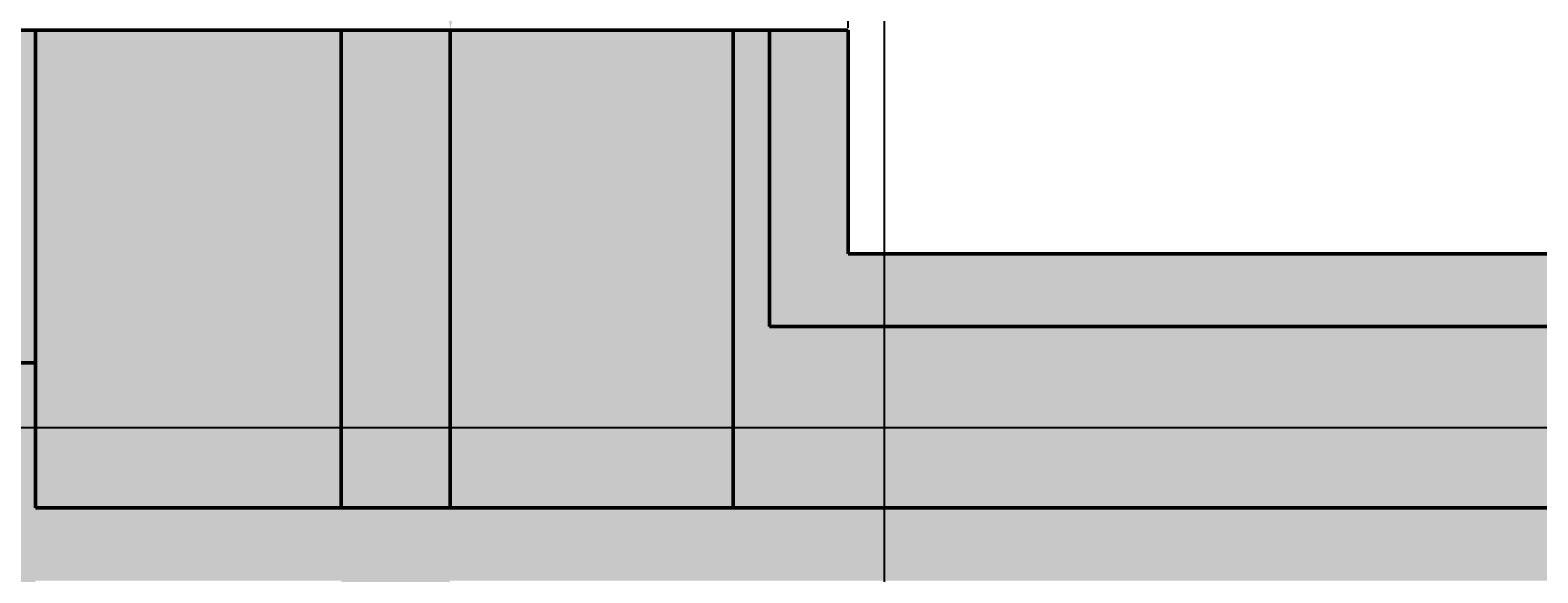
# Model space of a CAD drawing. Units: inches. Extents: x -12 to 334, y -10 to 186.
# Tile 19 of 77: x 64 to 106, y 94 to 109. Entities that reach past the tile are written whole.
import ezdxf
from ezdxf import colors
from ezdxf.entities.mleader import LeaderData, LeaderLine
from ezdxf.math import Vec2, Vec3

# ---------------------------------------------------------------- set-up
doc = ezdxf.new("R2010")
doc.units = ezdxf.units.IN
doc.header["$MEASUREMENT"] = 0
for name, color, linetype, lineweight in [('M-ANNO-TEXT', 3, 'Continuous', 25), ('M-DIMS', 2, 'Continuous', 18), ('M-EQPM', 7, 'Continuous', 50), ('M-EQPM-PATT', 8, 'Continuous', 18)]:
    doc.layers.add(name, color=color, linetype=linetype, lineweight=lineweight)
doc.styles.get("Standard").update_dxf_attribs({"font": 'arial.ttf'})
doc.dimstyles.get("Standard").update_dxf_attribs({"dimtxt": 0.18, "dimasz": 0.18, "dimexe": 0.18, "dimexo": 0.0625, "dimgap": 0.09, "dimtad": 0, "dimtih": 1, "dimtoh": 1, "dimdec": 4, "dimzin": 0, "dimdsep": 46, "dimtxsty": 'Standard', "dimcen": 0.09, "dimadec": 0, "dimazin": 0, "dimtfac": 1, "dimtdec": 4, "dimtofl": 0, "dimtmove": 0, "dimatfit": 3, "dimfxl": 1, "dimtolj": 1, "dimtzin": 0, "dimarcsym": 0})

# ---------------------------------------------------------------- blocks, each defined once
blk = doc.blocks.new('*D15')
at = {"layer": 'Defpoints', "color": 0, "transparency": 16777216}
for p in [(106.177, 169.385), (86.888, 109.058), (106.177, 102.896)]:
    blk.add_point(p, dxfattribs=at)
at = {"layer": 'M-DIMS', "color": 0, "lineweight": -2, "transparency": 16777216}
for p, q in [((86.888, 109.121), (86.888, 169.565)), ((106.177, 102.958), (106.177, 169.565)), ((87.068, 169.385), (96.147, 169.385)), ((105.997, 169.385), (96.918, 169.385))]:
    blk.add_line(p, q, dxfattribs=at)
at = {"layer": 'M-DIMS', "color": 0, "transparency": 16777216}
for points in [[(87.068, 169.415), (87.068, 169.355), (86.888, 169.385)], [(105.997, 169.415), (105.997, 169.355), (106.177, 169.385)]]:
    blk.add_solid(points, dxfattribs=at)
at = {"layer": 'M-DIMS', "color": 0, "transparency": 16777216, "insert": (96.532, 169.385), "char_height": 0.18, "attachment_point": 5}
blk.add_mtext('\\A1;19.29', dxfattribs=at)
blk = doc.blocks.new('*D26')
at = {"layer": 'Defpoints', "color": 0, "transparency": 16777216}
for p in [(87.888, 169.385), (87.888, 56.321), (58.1, 33.675)]:
    blk.add_point(p, dxfattribs=at)
at = {"layer": 'M-DIMS', "color": 0, "lineweight": -2, "transparency": 16777216}
for p, q in [((58.1, 33.738), (58.1, 169.565)), ((87.888, 56.383), (87.888, 169.565)), ((58.28, 169.385), (72.599, 169.385)), ((87.708, 169.385), (73.389, 169.385))]:
    blk.add_line(p, q, dxfattribs=at)
at = {"layer": 'M-DIMS', "color": 0, "transparency": 16777216}
for points in [[(58.28, 169.415), (58.28, 169.355), (58.1, 169.385)], [(87.708, 169.415), (87.708, 169.355), (87.888, 169.385)]]:
    blk.add_solid(points, dxfattribs=at)
at = {"layer": 'M-DIMS', "color": 0, "transparency": 16777216, "insert": (72.994, 169.385), "char_height": 0.18, "attachment_point": 5}
blk.add_mtext('\\A1;29.79', dxfattribs=at)
blk = doc.blocks.new('*D35')
at = {"layer": 'Defpoints', "color": 0, "transparency": 16777216}
for p in [(216.428, 98.108), (-11.174, 61.105), (216.428, 61.105)]:
    blk.add_point(p, dxfattribs=at)
at = {"layer": 'M-DIMS', "color": 0, "lineweight": -2, "transparency": 16777216}
for p, q in [((216.365, 98.108), (-11.354, 98.108)), ((-11.174, 97.928), (-11.174, 79.788)), ((-11.174, 61.285), (-11.174, 79.424)), ((216.365, 61.105), (-11.354, 61.105))]:
    blk.add_line(p, q, dxfattribs=at)
at = {"layer": 'M-DIMS', "color": 0, "transparency": 16777216}
for points in [[(-11.204, 97.928), (-11.144, 97.928), (-11.174, 98.108)], [(-11.204, 61.285), (-11.144, 61.285), (-11.174, 61.105)]]:
    blk.add_solid(points, dxfattribs=at)
at = {"layer": 'M-DIMS', "color": 0, "transparency": 16777216, "insert": (-11.174, 79.606), "char_height": 0.18, "attachment_point": 5}
blk.add_mtext('\\A1;37', dxfattribs=at)

msp = doc.modelspace()

# ---------------------------------------------------------------- hatches: boundary and pattern name
at = {"layer": 'M-EQPM-PATT'}
h = msp.add_hatch(color=256, dxfattribs=at)
h.set_gradient(color1=(99, 100, 102), color2=(99, 100, 102), tint=1)
h.paths.add_polyline_path([(126.9567, 136.8871), (179.7818, 136.8871), (180.0106, 137.8871), (126.3793, 137.8871), (106.1771, 102.8958), (86.8879, 102.8958), (86.8879, 109.0583), (84.7229, 109.0583), (84.7229, 100.8958), (106.1771, 100.8958)])
h.paths.add_polyline_path([(196.3421, 152.8345), (195.3421, 152.8345), (195.3421, 137.8871), (180.0106, 137.8871), (179.7818, 136.8871), (196.3421, 136.8871)])
h.paths.add_polyline_path([(215.0166, 152.8345), (214.0166, 152.8345), (214.0166, 136.9435), (268.3808, 136.9435, -0.2673785), (268.3808, 46.8541), (249.3759, 46.8541), (249.8485, 45.8541), (269.3808, 45.8541, 0.2615891), (269.3808, 137.9435), (215.0166, 137.9435)])
h = msp.add_hatch(color=256, dxfattribs=at)
h.set_gradient(color1=(99, 100, 102), color2=(99, 100, 102), tint=1)
h.paths.add_polyline_path([(4.3766, 80.754, -0.4132606), (23.5807, 99.8958), (37.1002, 99.8958), (37.1002, 127.7078), (32.1002, 127.7078), (32.1002, 125.2078), (36.1002, 125.2078), (36.1002, 100.8958), (23.5807, 100.8958, 1), (23.5807, 60.4872), (36.1002, 60.4872), (36.1002, 36.1752), (32.1002, 36.1752), (32.1002, 33.6752), (37.1002, 33.6752), (37.1002, 61.4872), (23.5807, 61.4872, -0.384914), (4.4744, 78.754), (72.9244, 78.754), (72.9244, 69.6117), (75.9244, 69.6117), (75.9244, 89.8963), (72.9244, 89.8963), (72.9244, 80.754)])
h.paths.add_polyline_path([(54.1002, 125.2078), (58.1002, 125.2078), (58.1002, 127.7078), (53.1002, 127.7078), (53.1002, 99.8958), (64.5, 99.8958), (64.5, 109.0583), (63.5, 109.0583), (63.5, 100.8958), (54.1002, 100.8958)], flags=17)
h.paths.add_polyline_path([(53.1002, 33.6752), (58.1002, 33.6752), (58.1002, 36.1752), (54.1002, 36.1752), (54.1002, 60.4872), (64.2068, 60.4872), (64.2068, 49.4497), (87.8879, 49.4497), (87.8879, 55.3205), (104.8919, 55.3205), (104.8919, 30.8541), (99.8919, 30.8541), (99.8919, 28.8541), (105.8919, 28.8541), (105.8919, 56.3205), (87.8879, 56.3205), (87.8879, 63.6117), (86.8879, 63.6117), (86.8879, 50.4497), (65.0061, 50.4497), (65.0061, 63.6117), (64.5, 63.6117), (64.5, 61.4872), (53.1002, 61.4872)])
h.paths.add_polyline_path([(121.8919, 28.8541), (121.8919, 30.8541), (116.8919, 30.8541), (116.8919, 45.8541), (209.6965, 45.8541), (209.9204, 46.8541), (115.8919, 46.8541), (115.8919, 28.8541)])
h.paths.add_polyline_path([(221.5761, 32.8541), (216.5761, 32.8541), (216.5761, 30.8541), (222.5761, 30.8541), (222.5761, 46.8541), (209.9204, 46.8541), (209.6965, 45.8541), (221.5761, 45.8541)])
h.paths.add_polyline_path([(233.5761, 45.8541), (249.8485, 45.8541), (249.3759, 46.8541), (232.5761, 46.8541), (232.5761, 30.8541), (238.5761, 30.8541), (238.5761, 32.8541), (233.5761, 32.8541)])
h = msp.add_hatch(color=256, dxfattribs=at)
h.set_gradient(color1=(205, 32, 39), color2=(205, 32, 39), tint=1)
h.paths.add_polyline_path([(64.5, 80.754), (64.5, 89.8963), (226.6083, 89.8963, -1), (226.6083, 69.6117), (64.5, 69.6117), (64.5, 78.754), (4.4744, 78.754, 0.384914), (23.5807, 61.4872), (37.1002, 61.4872), (37.1002, 33.6752), (53.1002, 33.6752), (53.1002, 61.4872), (64.5, 61.4872), (64.5, 63.6117), (226.6083, 63.6117, 1), (226.6083, 95.8963), (64.5, 95.8963), (64.5, 99.8958), (53.1002, 99.8958), (53.1002, 127.7078), (37.1002, 127.7078), (37.1002, 99.8958), (23.5807, 99.8958, 0.4132606), (4.3766, 80.754)])
h.paths.add_polyline_path([(64.5, 91.8963), (64.5, 93.8963), (226.6083, 93.8963, -1), (226.6083, 65.6117), (64.5, 65.6117), (64.5, 67.6117), (226.6083, 67.6117, 1), (226.6083, 91.8963)], flags=16)
h = msp.add_hatch(color=256, dxfattribs=at)
h.set_gradient(color1=(205, 32, 39), color2=(205, 32, 39), tint=1)
h.paths.add_polyline_path([(72.9244, 95.8963), (72.9244, 109.0583), (64.5, 109.0583), (64.5, 95.8963)])
h.paths.add_polyline_path([(72.9244, 80.754), (72.9244, 89.8963), (64.5, 89.8963), (64.5, 80.754)])
h.paths.add_polyline_path([(72.9244, 69.6117), (72.9244, 78.754), (64.5, 78.754), (64.5, 69.6117)])
h.paths.add_polyline_path([(72.9244, 50.4497), (72.9244, 63.6117), (65.0061, 63.6117), (65.0061, 50.4497)])
h = msp.add_hatch(color=256, dxfattribs=at)
h.set_gradient(color1=(99, 100, 102), color2=(99, 100, 102), tint=1)
h.paths.add_polyline_path([(72.9244, 95.8963), (75.9244, 95.8963), (75.9244, 109.0583), (72.9244, 109.0583)])
h.paths.add_polyline_path([(72.9244, 50.4497), (75.9244, 50.4497), (75.9244, 63.6117), (72.9244, 63.6117)])
h.paths.add_polyline_path([(75.9244, 91.8963), (75.9244, 93.8963), (72.9244, 93.8963), (72.9244, 91.8963)])
h.paths.add_polyline_path([(75.9244, 65.6117), (75.9244, 67.6117), (72.9244, 67.6117), (72.9244, 65.6117)])
h.paths.add_polyline_path([(129.093, 69.6117), (130.8573, 69.6117), (130.8573, 89.8963), (129.093, 89.8963)])
h.paths.add_polyline_path([(129.093, 98.1081), (129.093, 95.8963), (130.8573, 95.8963), (130.8573, 98.1081)])
h.paths.add_polyline_path([(130.8573, 61.1045), (130.8573, 63.6117), (129.093, 63.6117), (129.093, 61.1045)])
h.paths.add_polyline_path([(170.9079, 69.6117), (172.6722, 69.6117), (172.6722, 89.8963), (170.9079, 89.8963)])
h.paths.add_polyline_path([(172.6722, 95.8963), (172.6722, 98.1081), (170.9079, 98.1081), (170.9079, 95.8963)])
h.paths.add_polyline_path([(170.9079, 61.1045), (172.6722, 61.1045), (172.6722, 63.6117), (170.9079, 63.6117)])
h.paths.add_polyline_path([(218.1922, 63.6117), (216.4278, 63.6117), (216.4278, 61.1045), (218.1922, 61.1045)])
h.paths.add_polyline_path([(216.4278, 69.6117), (218.1922, 69.6117), (218.1922, 89.8963), (216.4278, 89.8963)])
h.paths.add_polyline_path([(216.4278, 95.8963), (218.1922, 95.8963), (218.1922, 98.1081), (216.4278, 98.1081)])
h = msp.add_hatch(color=256, dxfattribs=at)
h.set_gradient(color1=(94, 103, 175), color2=(94, 103, 175), tint=1)
h.paths.add_polyline_path([(129.093, 89.8963), (86.8879, 89.8963), (86.8879, 69.6117), (129.093, 69.6117)], flags=17)
h.paths.add_polyline_path([(170.9079, 89.8963), (130.8573, 89.8963), (130.8573, 69.6117), (170.9079, 69.6117)], flags=17)
h.paths.add_polyline_path([(216.4278, 89.8963), (172.6722, 89.8963), (172.6722, 69.6117), (216.4278, 69.6117)], flags=17)
h.paths.add_polyline_path([(245.9354, 82.6969), (247.9354, 82.6969), (247.9354, 46.8541), (268.3808, 46.8541, 0.0998398), (279.7263, 80.6915), (251.9801, 80.6915, 0.4142136), (231.7758, 100.8958), (84.7229, 100.8958), (84.7229, 109.0583), (83.7229, 109.0583), (83.7229, 95.8963), (129.093, 95.8963), (129.093, 98.1081), (130.8573, 98.1081), (130.8573, 95.8963), (170.9079, 95.8963), (170.9079, 98.1081), (172.6722, 98.1081), (172.6722, 95.8963), (216.4278, 95.8963), (216.4278, 98.1081), (218.1922, 98.1081), (218.1922, 95.8963), (226.6083, 95.8963, -1), (226.6083, 63.6117), (218.1922, 63.6117), (218.1922, 61.1045), (216.4278, 61.1045), (216.4278, 63.6117), (172.6722, 63.6117), (172.6722, 61.1045), (170.9079, 61.1045), (170.9079, 63.6117), (130.8573, 63.6117), (130.8573, 61.1045), (129.093, 61.1045), (129.093, 63.6117), (87.8879, 63.6117), (87.8879, 56.3205), (105.8919, 56.3205), (105.8919, 28.8541), (115.8919, 28.8541), (115.8919, 46.8541), (222.5761, 46.8541), (222.5761, 30.8541), (232.5761, 30.8541), (232.5761, 46.8541), (245.9354, 46.8541)])
h.paths.add_polyline_path([(86.8879, 89.8963), (75.9244, 89.8963), (75.9244, 69.6117), (86.8879, 69.6117)])
h.paths.add_polyline_path([(83.7229, 109.0583), (75.9244, 109.0583), (75.9244, 95.8963), (83.7229, 95.8963)])
h.paths.add_polyline_path([(226.6083, 89.8963), (218.1922, 89.8963), (218.1922, 69.6117), (226.6083, 69.6117, 1)], flags=17)
h = msp.add_hatch(color=256, dxfattribs=at)
h.set_gradient(color1=(0, 0, 255), color2=(0, 0, 255), tint=1)
h.paths.add_polyline_path([(84.7229, 100.8958), (84.7229, 109.0583), (83.7229, 109.0583), (83.7229, 95.8963), (129.093, 95.8963), (129.093, 98.1081), (130.8573, 98.1081), (130.8573, 95.8963), (170.9079, 95.8963), (170.9079, 98.1081), (172.6722, 98.1081), (172.6722, 95.8963), (216.4278, 95.8963), (216.4278, 98.1081), (218.1922, 98.1081), (218.1922, 95.8963), (226.6083, 95.8963, -1), (226.6083, 63.6117), (218.1922, 63.6117), (218.1922, 61.1045), (216.4278, 61.1045), (216.4278, 63.6117), (172.6722, 63.6117), (172.6722, 61.1045), (170.9079, 61.1045), (170.9079, 63.6117), (130.8573, 63.6117), (130.8573, 61.1045), (129.093, 61.1045), (129.093, 63.6117), (87.8879, 63.6117), (87.8879, 56.3205), (105.8919, 56.3205), (105.8919, 28.8541), (115.8919, 28.8541), (115.8919, 46.8541), (222.5761, 46.8541), (222.5761, 30.8541), (232.5761, 30.8541), (232.5761, 46.8541), (245.9354, 46.8541), (245.9354, 82.6969), (247.9354, 82.6969), (247.9354, 46.8541), (268.3808, 46.8541, 0.0998398), (279.7263, 80.6915), (251.9801, 80.6915, 0.4142136), (231.7758, 100.8958)])

# ---------------------------------------------------------------- linework, layer by layer
at = {"layer": 'M-EQPM'}
for p, q in [((63.5, 109.0583), (86.8879, 109.0583)), ((64.5, 95.8963), (64.5, 109.0583)), ((72.9244, 109.0583), (72.9244, 95.8963)), ((75.9244, 109.0583), (75.9244, 95.8963)), ((83.7229, 109.0583), (83.7229, 95.8963)), ((84.7229, 109.0583), (84.7229, 100.8958)), ((86.8879, 109.0583), (86.8879, 102.8958))]:
    msp.add_line(p, q, dxfattribs=at)
for points in [[(86.8879, 102.8958), (106.1771, 102.8958)], [(84.7229, 100.8958), (231.7758, 100.8958)], [(53.1002, 99.8958), (64.5, 99.8958)]]:
    msp.add_lwpolyline(points, dxfattribs=at)
msp.add_lwpolyline([(64.5, 63.6117), (226.6083, 63.6117, 1), (226.6083, 95.8963), (64.5, 95.8963)], format="xyb", dxfattribs=at)

# ---------------------------------------------------------------- dimensions: what is measured, and where the dimension line sits
at = {"layer": 'M-DIMS'}
for base, p1, p2, picture, middle in [((87.8879, 169.3845), (58.1002, 33.6752), (87.8879, 56.3205), '*D26', (72.9941, 169.3845)), ((106.1771, 169.3845), (86.8879, 109.0583), (106.1771, 102.8958), '*D15', (96.5325, 169.3845))]:
    dim = msp.add_linear_dim(base=base, p1=p1, p2=p2, dimstyle='Standard', override={"dimdec": 2, "dimlfac": 1, "dimrnd": 0, "dimzin": 0, "dimdsep": 46, "dimlunit": 2}, dxfattribs=at)
    dim.commit()
    dim.dimension.update_dxf_attribs({"geometry": picture, "text_midpoint": middle})
dim = msp.add_linear_dim(base=(-11.1736, 61.1045), p1=(216.4278, 98.1081), p2=(216.4278, 61.1045), angle=90, dimstyle='Standard', override={"dimdec": 0, "dimlfac": 1, "dimrnd": 0, "dimzin": 0, "dimdsep": 46, "dimlunit": 2}, dxfattribs=at)
dim.commit()
dim.dimension.update_dxf_attribs({"geometry": '*D35', "text_midpoint": (-11.1735, 79.6063)})

# ---------------------------------------------------------------- leaders
at = {"layer": 'M-ANNO-TEXT'}
ml = msp.add_multileader_mtext('Standard', dxfattribs=at)
ml.set_content('Tube plate', color=256)
ml.set_leader_properties()
ml.build(insert=Vec2(0, 0))
ml.multileader.update_dxf_attribs({"dogleg_length": 0.36, "arrow_head_size": 0.7})
ctx = ml.context
ctx.base_point, ctx.arrow_head_size, ctx.landing_gap_size, ctx.plane_origin = Vec3(95.9742, 157.4218), 0.7, 0.09, Vec3(31.4743, 171.7024)
notes = []
notes.append((ctx, [(0, (1, 1, 0), (78.5354, 157.4218), (1, 0), 17.4388, [(0, [(75.9244, 109.0583)], 0, [])])]))
ctx.mtext.insert, ctx.mtext.flow_direction = Vec3(96.0642, 159.9771), 5
for ctx, leaders in notes:
    for number, flags, end, landing, length, lines in leaders:
        leader = LeaderData()
        leader.index, (leader.has_last_leader_line, leader.has_dogleg_vector, leader.attachment_direction) = number, flags
        leader.last_leader_point, leader.dogleg_vector, leader.dogleg_length = Vec3(end), Vec3(landing), length
        for number, points, colour, breaks in lines:
            line = LeaderLine()
            line.index, line.vertices, line.color, line.breaks = number, Vec3.list(points), colors.encode_raw_color(colour), breaks
            leader.lines.append(line)
        ctx.leaders.append(leader)

doc.saveas('drawing.dxf')
